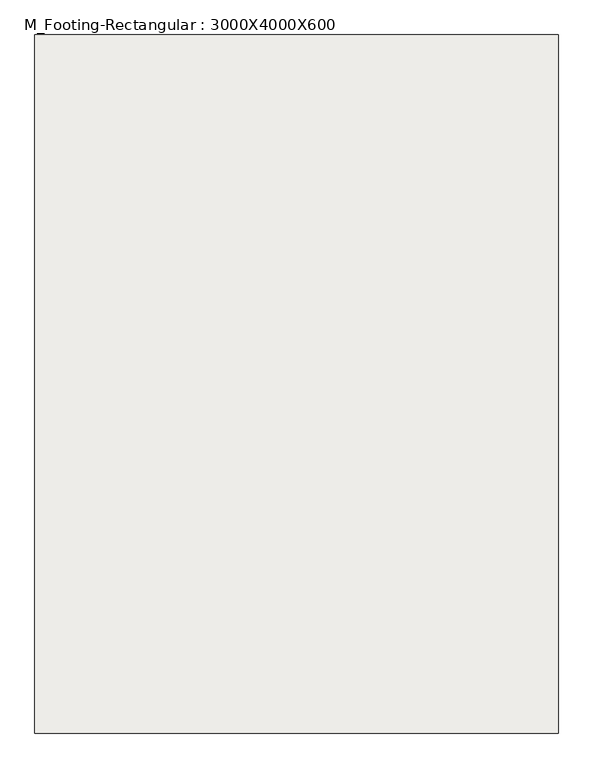
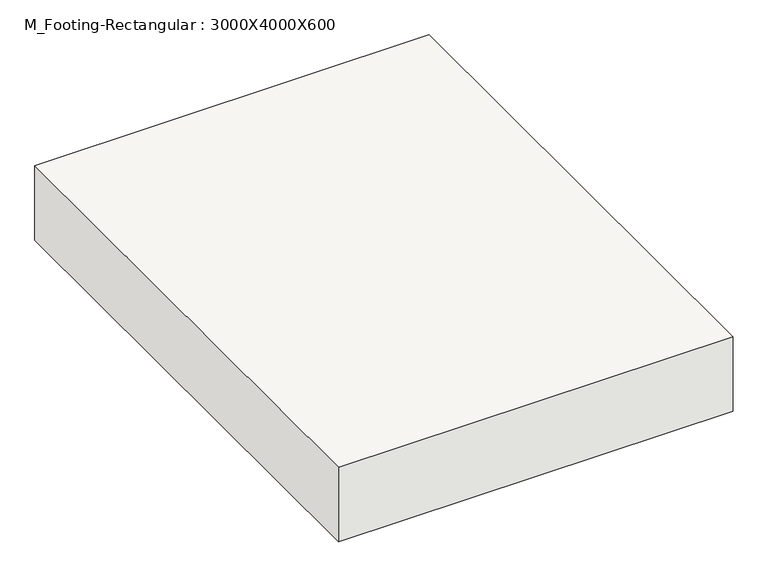
"""IFC4 building model written with IfcOpenShell, lengths in millimetres: slab geometry, M_Footing-Rectangular : 3000X4000X600."""

from ifc_helpers import new_model, si_unit, frame, origin, place, context, project, spatial, polyline, outline, extrude, source, transform, mapped, element, save


def m_footing_rectangular_3000x4000x600_f1bd0d4a(model_context):
    return source(origin(), model_context, "Body", "SweptSolid", [
        extrude(outline(polyline([(1500.0, 2000.0), (1500.0, -2000.0), (-1500.0, -2000.0), (-1500.0, 2000.0), (1500.0, 2000.0)])), frame((0.0, 0.0, -600.0), z_axis=(0.0, 0.0, 1.0), x_axis=(1.0, 0.0, 0.0)), (0.0, 0.0, 1.0), 600.0),
    ])


if __name__ == "__main__":
    model = new_model("IFC4")
    model_context = context("Model", 3, world=origin())
    ifc_project = project(units=[si_unit("LENGTHUNIT", "METRE", prefix="MILLI")], contexts=[model_context])
    site = spatial("IfcSite", under=ifc_project)
    building = spatial("IfcBuilding", under=site)
    placement = place(None, origin())
    m_footing_rectangular_3000x4000x600_shape = m_footing_rectangular_3000x4000x600_f1bd0d4a(model_context)
    element("IfcSlab", 1, ObjectType="M_Footing-Rectangular : 3000X4000X600", at=placement, inside=building, context=model_context, shape_type="MappedRepresentation", body=[
        mapped(m_footing_rectangular_3000x4000x600_shape, transform((0.0, 0.0, 0.0), x_axis=(1.0, 0.0, 0.0), y_axis=(0.0, 1.0, 0.0), z_axis=(0.0, 0.0, 1.0))),
    ])
    save(model, "model.ifc")

# Revit data of these elements
# Type "M_Footing-Rectangular : 3000X4000X600"
#   Width = 3000 mm
#   Length = 4000 mm
#   Foundation Thickness = 600 mm
#   Structural Material [instance default] = Concrete, Cast-in-Place gray
#   Assembly Code = ""
# Element 1 (IfcSlab, "M_Footing-Rectangular : 3000X4000X600")
#   Structural Material = Concrete, Cast In Situ
#   Materials on its faces: "Concrete, Cast In Situ"
# Materials
#   "Concrete, Cast-in-Place gray": class "Concrete", colour RGB 192 192 192, transparency 0, Description = "Cast-in-place concrete", Cost = 0
#   "Concrete, Cast In Situ": class "Concrete", colour RGB 192 192 192, transparency 0, Description = "physical material", Cost = 0
